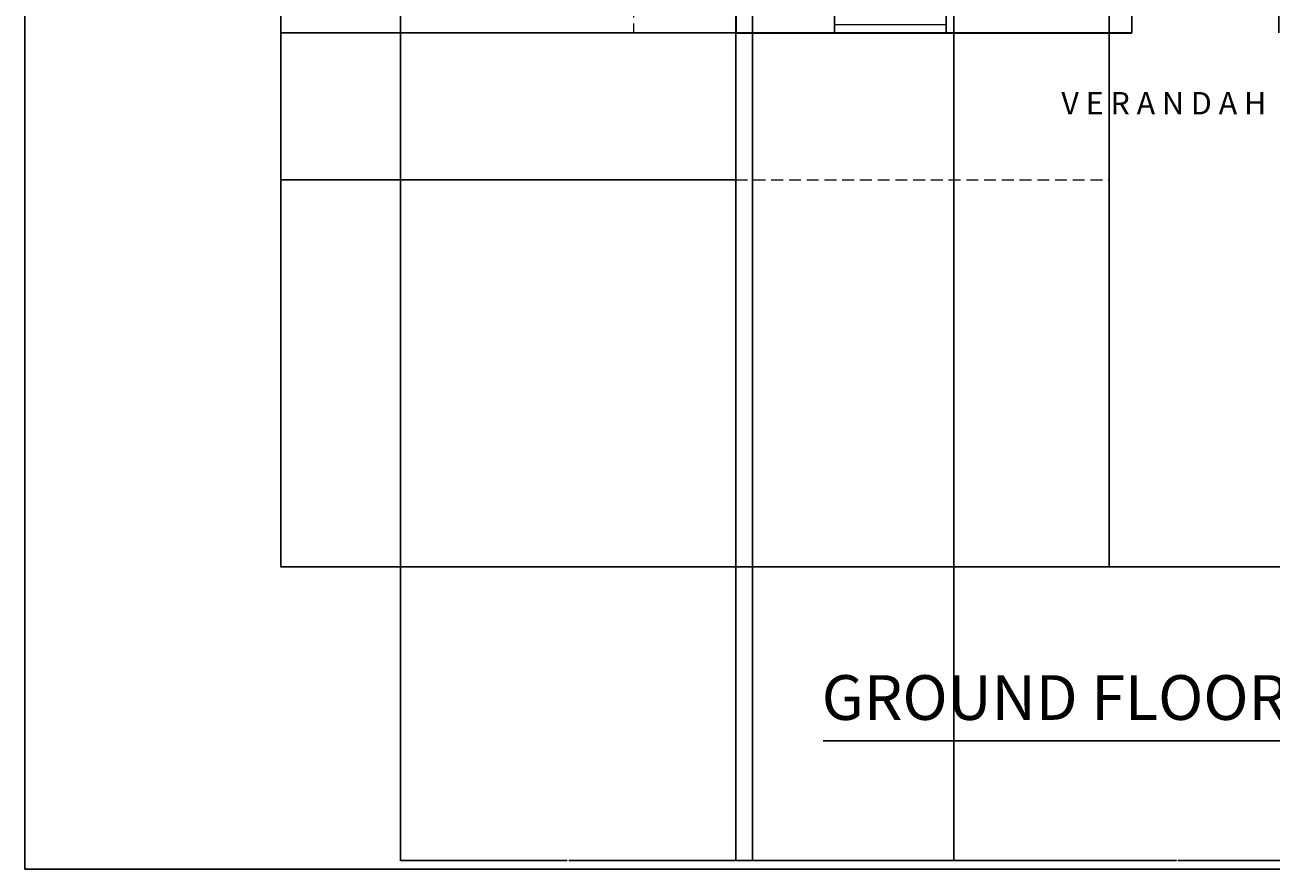
# Model space of a CAD drawing. Units: inches. Extents: x 1770 to 2988, y 1161 to 3221.
# Tile 1 of 44: x 1770 to 2439, y 1161 to 1614. Entities that reach past the tile are written whole.
import ezdxf

# ---------------------------------------------------------------- set-up
doc = ezdxf.new("R2010")
doc.units = ezdxf.units.IN
doc.linetypes.add('DASHED2', pattern=[9.525, 6.35, -3.175])
for name, color, linetype, lineweight in [('A-ANNO-DIMS', 2, 'Continuous', 18), ('A-ANNO-TEXT', 7, 'Continuous', 25), ('A-ANNO-TTLB', 7, 'Continuous', 25), ('A-AREA-IDEN', 7, 'Continuous', 18), ('A-DOOR', 4, 'Continuous', 18), ('A-GLAZ', 4, 'Continuous', 18), ('A-ROOF-OVHD', 7, 'DASHED2', 18), ('A-WALL', 7, 'Continuous', 35), ('C-PROP', 7, 'Continuous', 25), ('C-SITE-PAVE', 8, 'Continuous', 18)]:
    doc.layers.add(name, color=color, linetype=linetype, lineweight=lineweight)
doc.styles.get("Standard").update_dxf_attribs({"font": 'arial.ttf'})
doc.dimstyles.get("Standard").update_dxf_attribs({"dimtxt": 0.18, "dimasz": 0.18, "dimexe": 0.18, "dimexo": 0.0625, "dimgap": 0.09, "dimtad": 0, "dimtih": 1, "dimtoh": 1, "dimdec": 4, "dimzin": 0, "dimdsep": 46, "dimtxsty": 'Standard', "dimcen": 0.09, "dimadec": 0, "dimazin": 0, "dimtfac": 1, "dimtdec": 4, "dimtofl": 0, "dimtmove": 0, "dimatfit": 3, "dimfxl": 1, "dimtolj": 1, "dimtzin": 0, "dimarcsym": 0})

# ---------------------------------------------------------------- blocks, each defined once
blk = doc.blocks.new('WIN-60-EXT')
for p, q in [((0, 9), (0, 0)), ((60, 4.5), (60, 9)), ((60, 9), (60, 0)), ((0, 0), (0, 4.5)), ((0, 4.5), (60, 4.5))]:
    blk.add_line(p, q)
blk = doc.blocks.new('*D57')
at = {"layer": 'A-ANNO-DIMS', "color": 0, "lineweight": -2, "transparency": 16777216}
for p, q in [((1971.47, 2506.27), (1907.1, 2506.27)), ((1907.28, 2506.09), (1907.28, 1915.08)), ((1907.28, 1323.71), (1907.28, 1914.72)), ((1971.47, 1323.53), (1907.1, 1323.53))]:
    blk.add_line(p, q, dxfattribs=at)
at = {"layer": 'A-ANNO-DIMS', "color": 0, "transparency": 16777216}
for points in [[(1907.25, 2506.09), (1907.31, 2506.09), (1907.28, 2506.27)], [(1907.25, 1323.71), (1907.31, 1323.71), (1907.28, 1323.53)]]:
    blk.add_solid(points, dxfattribs=at)
at = {"layer": 'Defpoints', "color": 0, "transparency": 16777216}
for p in [(1907.28, 2506.27), (1971.53, 2506.27), (1971.53, 1323.53)]:
    blk.add_point(p, dxfattribs=at)
at = {"layer": 'A-ANNO-DIMS', "color": 0, "transparency": 16777216, "insert": (1907.28, 1914.9), "char_height": 0.18, "attachment_point": 5}
blk.add_mtext('\\A1;1182.7', dxfattribs=at)
blk = doc.blocks.new('*D58')
at = {"layer": 'A-ANNO-DIMS', "color": 0, "lineweight": -2, "transparency": 16777216}
for p, q in [((2151.7, 1610.14), (2151.7, 1165.57)), ((1971.53, 1323.47), (1971.53, 1165.57)), ((1971.71, 1165.75), (2061.16, 1165.75)), ((2151.52, 1165.75), (2062.07, 1165.75))]:
    blk.add_line(p, q, dxfattribs=at)
at = {"layer": 'A-ANNO-DIMS', "color": 0, "transparency": 16777216}
for points in [[(1971.71, 1165.78), (1971.71, 1165.72), (1971.53, 1165.75)], [(2151.52, 1165.78), (2151.52, 1165.72), (2151.7, 1165.75)]]:
    blk.add_solid(points, dxfattribs=at)
at = {"layer": 'Defpoints', "color": 0, "transparency": 16777216}
for p in [(2151.7, 1610.2), (1971.53, 1323.53), (2151.7, 1165.75)]:
    blk.add_point(p, dxfattribs=at)
at = {"layer": 'A-ANNO-DIMS', "color": 0, "transparency": 16777216, "insert": (2061.62, 1165.75), "char_height": 0.18, "attachment_point": 5}
blk.add_mtext('\\A1;180.16', dxfattribs=at)
blk = doc.blocks.new('*D60')
at = {"layer": 'A-ANNO-DIMS', "color": 0, "lineweight": -2, "transparency": 16777216}
for p, q in [((2151.7, 1610.14), (2151.7, 1165.57)), ((2625.7, 1610.14), (2625.7, 1165.57)), ((2151.88, 1165.75), (2388.4, 1165.75)), ((2625.52, 1165.75), (2388.99, 1165.75))]:
    blk.add_line(p, q, dxfattribs=at)
at = {"layer": 'A-ANNO-DIMS', "color": 0, "transparency": 16777216}
for points in [[(2151.88, 1165.78), (2151.88, 1165.72), (2151.7, 1165.75)], [(2625.52, 1165.78), (2625.52, 1165.72), (2625.7, 1165.75)]]:
    blk.add_solid(points, dxfattribs=at)
at = {"layer": 'Defpoints', "color": 0, "transparency": 16777216}
for p in [(2151.7, 1610.2), (2625.7, 1610.2), (2625.7, 1165.75)]:
    blk.add_point(p, dxfattribs=at)
at = {"layer": 'A-ANNO-DIMS', "color": 0, "transparency": 16777216, "insert": (2388.7, 1165.75), "char_height": 0.18, "attachment_point": 5}
blk.add_mtext('\\A1;474', dxfattribs=at)
blk = doc.blocks.new('*D62')
at = {"layer": 'A-ANNO-DIMS', "color": 0, "lineweight": -2, "transparency": 16777216}
for p, q in [((2151.63, 1610.2), (1907.1, 1610.2)), ((1907.28, 1610.02), (1907.28, 1570.95)), ((1907.28, 1531.52), (1907.28, 1570.59)), ((2151.63, 1531.34), (1907.1, 1531.34))]:
    blk.add_line(p, q, dxfattribs=at)
at = {"layer": 'A-ANNO-DIMS', "color": 0, "transparency": 16777216}
for points in [[(1907.25, 1610.02), (1907.31, 1610.02), (1907.28, 1610.2)], [(1907.25, 1531.52), (1907.31, 1531.52), (1907.28, 1531.34)]]:
    blk.add_solid(points, dxfattribs=at)
at = {"layer": 'Defpoints', "color": 0, "transparency": 16777216}
for p in [(1907.28, 1610.2), (2151.7, 1610.2), (2151.7, 1531.34)]:
    blk.add_point(p, dxfattribs=at)
at = {"layer": 'A-ANNO-DIMS', "color": 0, "transparency": 16777216, "insert": (1907.28, 1570.77), "char_height": 0.18, "attachment_point": 5}
blk.add_mtext('\\A1;78.86', dxfattribs=at)
blk = doc.blocks.new('*D63')
at = {"layer": 'A-ANNO-DIMS', "color": 0, "lineweight": -2, "transparency": 16777216}
for p, q in [((2352.17, 1323.59), (2352.17, 2570.7)), ((2352.35, 2570.52), (2401.24, 2570.52)), ((2450.91, 2570.52), (2402.02, 2570.52)), ((2451.09, 1323.59), (2451.09, 2570.7))]:
    blk.add_line(p, q, dxfattribs=at)
at = {"layer": 'A-ANNO-DIMS', "color": 0, "transparency": 16777216}
for points in [[(2352.35, 2570.55), (2352.35, 2570.49), (2352.17, 2570.52)], [(2450.91, 2570.55), (2450.91, 2570.49), (2451.09, 2570.52)]]:
    blk.add_solid(points, dxfattribs=at)
at = {"layer": 'Defpoints', "color": 0, "transparency": 16777216}
for p in [(2451.09, 2570.52), (2352.17, 1323.53), (2451.09, 1323.53)]:
    blk.add_point(p, dxfattribs=at)
at = {"layer": 'A-ANNO-DIMS', "color": 0, "transparency": 16777216, "insert": (2401.63, 2570.52), "char_height": 0.18, "attachment_point": 5}
blk.add_mtext('\\A1;98.93', dxfattribs=at)
blk = doc.blocks.new('*D70')
at = {"layer": 'A-ANNO-DIMS', "color": 0, "lineweight": -2, "transparency": 16777216}
for p, q in [((2160.7, 2171.14), (2160.7, 1165.57)), ((2268.7, 2171.14), (2268.7, 1165.57)), ((2160.88, 1165.75), (2214.42, 1165.75)), ((2268.52, 1165.75), (2214.98, 1165.75))]:
    blk.add_line(p, q, dxfattribs=at)
at = {"layer": 'A-ANNO-DIMS', "color": 0, "transparency": 16777216}
for points in [[(2160.88, 1165.78), (2160.88, 1165.72), (2160.7, 1165.75)], [(2268.52, 1165.78), (2268.52, 1165.72), (2268.7, 1165.75)]]:
    blk.add_solid(points, dxfattribs=at)
at = {"layer": 'Defpoints', "color": 0, "transparency": 16777216}
for p in [(2160.7, 2171.2), (2268.7, 2171.2), (2268.7, 1165.75)]:
    blk.add_point(p, dxfattribs=at)
at = {"layer": 'A-ANNO-DIMS', "color": 0, "transparency": 16777216, "insert": (2214.7, 1165.75), "char_height": 0.18, "attachment_point": 5}
blk.add_mtext('\\A1;108', dxfattribs=at)
blk = doc.blocks.new('*D79')
at = {"layer": 'A-ANNO-DIMS', "color": 0, "lineweight": -2, "transparency": 16777216}
for p, q in [((2151.7, 1610.26), (2151.7, 2570.7)), ((2151.88, 2570.52), (2177.78, 2570.52)), ((2204.48, 2570.52), (2178.57, 2570.52)), ((2204.66, 1610.26), (2204.66, 2570.7))]:
    blk.add_line(p, q, dxfattribs=at)
at = {"layer": 'A-ANNO-DIMS', "color": 0, "transparency": 16777216}
for points in [[(2151.88, 2570.55), (2151.88, 2570.49), (2151.7, 2570.52)], [(2204.48, 2570.55), (2204.48, 2570.49), (2204.66, 2570.52)]]:
    blk.add_solid(points, dxfattribs=at)
at = {"layer": 'Defpoints', "color": 0, "transparency": 16777216}
for p in [(2204.66, 2570.52), (2151.7, 1610.2), (2204.66, 1610.2)]:
    blk.add_point(p, dxfattribs=at)
at = {"layer": 'A-ANNO-DIMS', "color": 0, "transparency": 16777216, "insert": (2178.18, 2570.52), "char_height": 0.18, "attachment_point": 5}
blk.add_mtext('\\A1;52.96', dxfattribs=at)
blk = doc.blocks.new('*D80')
at = {"layer": 'A-ANNO-DIMS', "color": 0, "lineweight": -2, "transparency": 16777216}
for p, q in [((2264.66, 1610.26), (2264.66, 2570.7)), ((2264.84, 2570.52), (2314.14, 2570.52)), ((2364.23, 2570.52), (2314.93, 2570.52)), ((2364.41, 1610.26), (2364.41, 2570.7))]:
    blk.add_line(p, q, dxfattribs=at)
at = {"layer": 'A-ANNO-DIMS', "color": 0, "transparency": 16777216}
for points in [[(2264.84, 2570.55), (2264.84, 2570.49), (2264.66, 2570.52)], [(2364.23, 2570.55), (2364.23, 2570.49), (2364.41, 2570.52)]]:
    blk.add_solid(points, dxfattribs=at)
at = {"layer": 'Defpoints', "color": 0, "transparency": 16777216}
for p in [(2364.41, 2570.52), (2264.66, 1610.2), (2364.41, 1610.2)]:
    blk.add_point(p, dxfattribs=at)
at = {"layer": 'A-ANNO-DIMS', "color": 0, "transparency": 16777216, "insert": (2314.53, 2570.52), "char_height": 0.18, "attachment_point": 5}
blk.add_mtext('\\A1;99.76', dxfattribs=at)
blk = doc.blocks.new('*D81')
at = {"layer": 'A-ANNO-DIMS', "color": 0, "lineweight": -2, "transparency": 16777216}
for p, q in [((2364.41, 1610.26), (2364.41, 2570.7)), ((2364.59, 2570.52), (2403.51, 2570.52)), ((2443.21, 2570.52), (2404.29, 2570.52)), ((2443.39, 1610.26), (2443.39, 2570.7))]:
    blk.add_line(p, q, dxfattribs=at)
at = {"layer": 'A-ANNO-DIMS', "color": 0, "transparency": 16777216}
for points in [[(2364.59, 2570.55), (2364.59, 2570.49), (2364.41, 2570.52)], [(2443.21, 2570.55), (2443.21, 2570.49), (2443.39, 2570.52)]]:
    blk.add_solid(points, dxfattribs=at)
at = {"layer": 'Defpoints', "color": 0, "transparency": 16777216}
for p in [(2443.39, 2570.52), (2364.41, 1610.2), (2443.39, 1610.2)]:
    blk.add_point(p, dxfattribs=at)
at = {"layer": 'A-ANNO-DIMS', "color": 0, "transparency": 16777216, "insert": (2403.9, 2570.52), "char_height": 0.18, "attachment_point": 5}
blk.add_mtext('\\A1;78.97', dxfattribs=at)

msp = doc.modelspace()

# ---------------------------------------------------------------- linework, layer by layer
at = {"layer": 'A-ANNO-TEXT'}
msp.add_line((2198.6214, 1230.002), (2566.3223, 1230.002), dxfattribs=at)
at = {"layer": 'A-ANNO-TTLB'}
msp.add_lwpolyline([(1769.9155, 3221.2788), (2987.7567, 3221.2788), (2987.7567, 1161.1516), (1769.9155, 1161.1516)], close=True, dxfattribs=at)
at = {"layer": 'A-DOOR'}
for p, q in [((2364.4122, 1619.2021), (2364.4122, 1610.2021)), ((2364.4122, 1610.2021), (2364.4122, 1614.7021))]:
    msp.add_line(p, q, dxfattribs=at)
at = {"layer": 'A-ROOF-OVHD'}
for p, q in [((2096.7313, 2405.7876), (2096.7313, 1610.2021)), ((2096.7313, 1610.2021), (2151.696, 1610.2021)), ((2151.696, 1610.2021), (2151.696, 1531.3388)), ((2151.696, 1531.3388), (2352.1672, 1531.3388))]:
    msp.add_line(p, q, dxfattribs=at)
at = {"layer": 'A-WALL'}
for p, q in [((2151.696, 2376.7021), (2151.696, 1610.2021)), ((2151.696, 1610.2021), (2364.4122, 1610.2021))]:
    msp.add_line(p, q, dxfattribs=at)
at = {"layer": 'C-PROP'}
msp.add_lwpolyline([(1971.5344, 2506.2747), (2802.4374, 2506.2747), (2802.4374, 1323.5288), (1971.5344, 1323.5288)], close=True, dxfattribs=at)
at = {"layer": 'C-SITE-PAVE'}
msp.add_line((2352.1672, 1531.3388), (2352.1672, 1323.5288), dxfattribs=at)

# ---------------------------------------------------------------- block references
at = {"layer": 'A-GLAZ'}
msp.add_blockref('WIN-60-EXT', (2204.657, 1610.202), dxfattribs=at)

# ---------------------------------------------------------------- texts
at = {"layer": 'A-ANNO-TEXT', "insert": (2197.8268, 1265.2621), "char_height": 24, "attachment_point": 1}
msp.add_mtext_dynamic_manual_height_columns('GROUND FLOOR PLAN', width=505.43924, gutter_width=12.5, heights=[0], dxfattribs=at)
at = {"layer": 'A-AREA-IDEN', "insert": (2326.4899, 1578.4392), "char_height": 12, "attachment_point": 1}
msp.add_mtext_dynamic_manual_height_columns('V E R A N D A H', width=200.505816, gutter_width=12.5, heights=[0], dxfattribs=at)

# ---------------------------------------------------------------- dimensions: what is measured, and where the dimension line sits
at = {"layer": 'A-ANNO-DIMS'}
for base, p1, p2, override, picture, middle in [((2204.6568, 2570.5247), (2151.696, 1610.2021), (2204.6568, 1610.2021), {"dimdec": 2, "dimlfac": 1, "dimrnd": 0, "dimzin": 0, "dimdsep": 46, "dimlunit": 2}, '*D79', (2178.1764, 2570.5247)), ((2364.4122, 2570.5247), (2264.6568, 1610.2021), (2364.4122, 1610.2021), {"dimdec": 2, "dimlfac": 1, "dimrnd": 0, "dimzin": 0, "dimdsep": 46, "dimlunit": 2}, '*D80', (2314.5345, 2570.5247)), ((2451.0947, 2570.5247), (2352.1672, 1323.5288), (2451.0947, 1323.5288), {"dimdec": 2, "dimlfac": 1, "dimrnd": 0, "dimzin": 0, "dimdsep": 46, "dimlunit": 2}, '*D63', (2401.631, 2570.5247)), ((2443.3863, 2570.5247), (2364.4122, 1610.2021), (2443.3863, 1610.2021), {"dimdec": 2, "dimlfac": 1, "dimrnd": 0, "dimzin": 0, "dimdsep": 46, "dimlunit": 2}, '*D81', (2403.8993, 2570.5247)), ((2268.696, 1165.752), (2160.696, 2171.2021), (2268.696, 2171.2021), {"dimdec": 0, "dimlfac": 1, "dimrnd": 0, "dimzin": 0, "dimdsep": 46, "dimlunit": 2}, '*D70', (2214.696, 1165.752)), ((2151.696, 1165.752), (1971.5344, 1323.5288), (2151.696, 1610.2021), {"dimdec": 2, "dimlfac": 1, "dimrnd": 0, "dimzin": 0, "dimdsep": 46, "dimlunit": 2}, '*D58', (2061.6152, 1165.752)), ((2625.696, 1165.752), (2151.696, 1610.2021), (2625.696, 1610.2021), {"dimdec": 0, "dimlfac": 1, "dimrnd": 0, "dimzin": 0, "dimdsep": 46, "dimlunit": 2}, '*D60', (2388.696, 1165.752))]:
    dim = msp.add_linear_dim(base=base, p1=p1, p2=p2, dimstyle='Standard', override=override, dxfattribs=at)
    dim.commit()
    dim.dimension.update_dxf_attribs({"geometry": picture, "text_midpoint": middle})
for base, p1, p2, override, picture, middle in [((1907.2844, 2506.2747), (1971.5344, 1323.5288), (1971.5344, 2506.2747), {"dimdec": 1, "dimlfac": 1, "dimrnd": 0, "dimzin": 0, "dimdsep": 46, "dimlunit": 2}, '*D57', (1907.2844, 1914.9017)), ((1907.2844, 1610.2021), (2151.696, 1531.3388), (2151.696, 1610.2021), {"dimdec": 2, "dimlfac": 1, "dimrnd": 0, "dimzin": 0, "dimdsep": 46, "dimlunit": 2}, '*D62', (1907.2844, 1570.7705))]:
    dim = msp.add_linear_dim(base=base, p1=p1, p2=p2, angle=90, dimstyle='Standard', override=override, dxfattribs=at)
    dim.commit()
    dim.dimension.update_dxf_attribs({"geometry": picture, "text_midpoint": middle})

doc.saveas('drawing.dxf')
